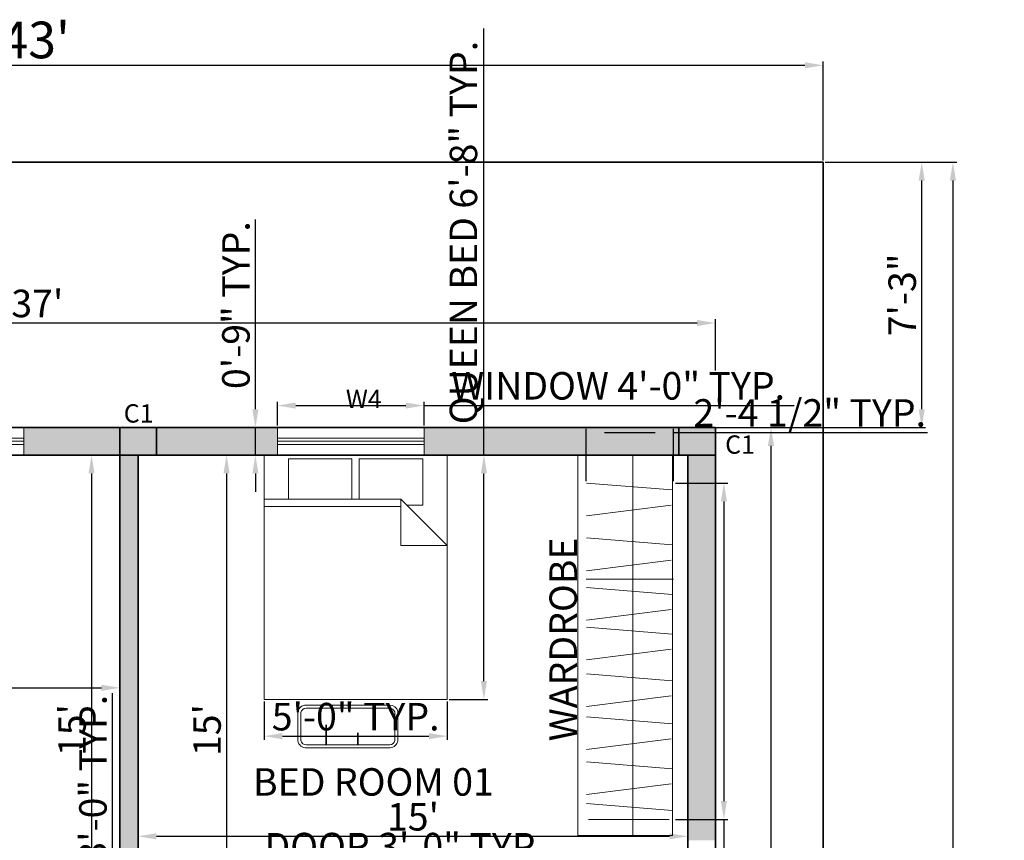
# Model space of a CAD drawing. Units: inches. Extents: x 4312 to 4955, y 6030 to 6717.
# Tile 5 of 5: x 4632 to 4955, y 6418 to 6686. Entities that reach past the tile are written whole.
import ezdxf

# ---------------------------------------------------------------- set-up
doc = ezdxf.new("R2010")
doc.units = ezdxf.units.IN
for name, color, linetype, lineweight in [('A-AREA-IDEN', 7, 'Continuous', 20), ('A-FLOR-CASE', 40, 'Continuous', 18), ('A-WALL', 7, 'Continuous', 35), ('C-PROP', 7, 'Continuous', 35), ('Dimensions', 112, 'Continuous', 13), ('Furniture', 30, 'Continuous', 18), ('Text', 30, 'Continuous', 18), ('Windows', 160, 'Continuous', 18)]:
    doc.layers.add(name, color=color, linetype=linetype, lineweight=lineweight)
doc.layers.add('A-WALL-PATT', color=251, linetype='Continuous', lineweight=13, true_color=0x636466)
doc.layers.add('Column', color=52, linetype='Continuous', lineweight=35, true_color=0xc8c92d)
doc.styles.get("Standard").update_dxf_attribs({"font": 'arial.ttf'})
doc.dimstyles.new('ISO-25', dxfattribs={"dimtxt": 9, "dimasz": 6, "dimexe": 1.25, "dimexo": 0.625, "dimtad": 1, "dimdec": 1, "dimlunit": 3, "dimtxsty": 'Standard', "dimcen": 2.5, "dimadec": 0, "dimazin": 0, "dimtfac": 1, "dimtdec": 1, "dimtmove": 0, "dimatfit": 3, "dimfxl": 1, "dimarcsym": 0})

# ---------------------------------------------------------------- blocks, each defined once
blk = doc.blocks.new('W')
at = {"layer": 'Windows'}
for p, q in [((4457.75, 6177.72), (4457.75, 6168.72)), ((4505.75, 6177.72), (4505.75, 6168.72)), ((4457.75, 6174.22), (4505.75, 6174.22)), ((4457.75, 6173.22), (4505.75, 6173.22)), ((4457.75, 6172.22), (4505.75, 6172.22))]:
    blk.add_line(p, q, dxfattribs=at)
blk = doc.blocks.new('*D11')
at = {"layer": 'Defpoints', "color": 0, "transparency": 16777216}
for p in [(4551.05, 6471.59), (4665.05, 6471.59), (4665.05, 6467.55)]:
    blk.add_point(p, dxfattribs=at)
at = {"layer": 'Dimensions', "color": 0, "lineweight": -2, "transparency": 16777216}
for p, q in [((4551.05, 6470.96), (4551.05, 6466.3)), ((4665.05, 6470.96), (4665.05, 6466.3)), ((4557.05, 6467.55), (4659.05, 6467.55))]:
    blk.add_line(p, q, dxfattribs=at)
at = {"layer": 'Dimensions', "color": 0, "transparency": 16777216}
for points in [[(4557.05, 6468.55), (4557.05, 6466.55), (4551.05, 6467.55)], [(4659.05, 6468.55), (4659.05, 6466.55), (4665.05, 6467.55)]]:
    blk.add_solid(points, dxfattribs=at)
at = {"layer": 'Dimensions', "color": 0, "transparency": 16777216, "insert": (4608.05, 6472.77), "char_height": 9, "attachment_point": 5}
blk.add_mtext('9\'-6"', dxfattribs=at)
blk = doc.blocks.new('*D12')
at = {"layer": 'Defpoints', "color": 0, "transparency": 16777216}
for p in [(4655.8, 6543.72), (4655.8, 6363.72), (4665.05, 6363.72)]:
    blk.add_point(p, dxfattribs=at)
at = {"layer": 'Dimensions', "color": 0, "lineweight": -2, "transparency": 16777216}
for p, q in [((4656.43, 6543.72), (4657.05, 6543.72)), ((4655.8, 6537.72), (4655.8, 6369.72)), ((4664.42, 6363.72), (4654.55, 6363.72))]:
    blk.add_line(p, q, dxfattribs=at)
at = {"layer": 'Dimensions', "color": 0, "transparency": 16777216}
for points in [[(4654.8, 6537.72), (4656.8, 6537.72), (4655.8, 6543.72)], [(4654.8, 6369.72), (4656.8, 6369.72), (4655.8, 6363.72)]]:
    blk.add_solid(points, dxfattribs=at)
at = {"layer": 'Dimensions', "color": 0, "transparency": 16777216, "insert": (4650.58, 6453.72), "char_height": 9, "attachment_point": 5, "rotation": 90}
blk.add_mtext("15'", dxfattribs=at)
blk = doc.blocks.new('*D13')
at = {"layer": 'Defpoints', "color": 0, "transparency": 16777216}
for p in [(4690.28, 6543.72), (4690.28, 6363.72), (4700.01, 6363.72)]:
    blk.add_point(p, dxfattribs=at)
at = {"layer": 'Dimensions', "color": 0, "lineweight": -2, "transparency": 16777216}
for p, q in [((4690.91, 6543.72), (4701.26, 6543.72)), ((4700.01, 6537.72), (4700.01, 6369.72)), ((4690.91, 6363.72), (4701.26, 6363.72))]:
    blk.add_line(p, q, dxfattribs=at)
at = {"layer": 'Dimensions', "color": 0, "transparency": 16777216}
for points in [[(4699.01, 6537.72), (4701.01, 6537.72), (4700.01, 6543.72)], [(4699.01, 6369.72), (4701.01, 6369.72), (4700.01, 6363.72)]]:
    blk.add_solid(points, dxfattribs=at)
at = {"layer": 'Dimensions', "color": 0, "transparency": 16777216, "insert": (4694.79, 6453.72), "char_height": 9, "attachment_point": 5, "rotation": 90}
blk.add_mtext("15'", dxfattribs=at)
blk = doc.blocks.new('*D14')
at = {"layer": 'Defpoints', "color": 0, "transparency": 16777216}
for p in [(4671.05, 6418.94), (4851.05, 6418.94), (4851.05, 6418.94)]:
    blk.add_point(p, dxfattribs=at)
at = {"layer": 'Dimensions', "color": 0, "lineweight": -2, "transparency": 16777216}
for p, q in [((4671.05, 6419.56), (4671.05, 6420.19)), ((4677.05, 6418.94), (4845.05, 6418.94)), ((4851.05, 6419.56), (4851.05, 6420.19))]:
    blk.add_line(p, q, dxfattribs=at)
at = {"layer": 'Dimensions', "color": 0, "transparency": 16777216}
for points in [[(4677.05, 6419.94), (4677.05, 6417.94), (4671.05, 6418.94)], [(4845.05, 6419.94), (4845.05, 6417.94), (4851.05, 6418.94)]]:
    blk.add_solid(points, dxfattribs=at)
at = {"layer": 'Dimensions', "color": 0, "transparency": 16777216, "insert": (4761.05, 6424.16), "char_height": 9, "attachment_point": 5}
blk.add_mtext("15'", dxfattribs=at)
blk = doc.blocks.new('*D38')
at = {"layer": 'Defpoints', "color": 0, "transparency": 16777216}
for p in [(4860.05, 6586.94), (4416.05, 6570.77), (4860.05, 6570.77)]:
    blk.add_point(p, dxfattribs=at)
at = {"layer": 'Dimensions', "color": 0, "lineweight": -2, "transparency": 16777216}
for p, q in [((4416.05, 6571.39), (4416.05, 6588.19)), ((4422.05, 6586.94), (4854.05, 6586.94)), ((4860.05, 6571.39), (4860.05, 6588.19))]:
    blk.add_line(p, q, dxfattribs=at)
at = {"layer": 'Dimensions', "color": 0, "transparency": 16777216}
for points in [[(4422.05, 6587.94), (4422.05, 6585.94), (4416.05, 6586.94)], [(4854.05, 6587.94), (4854.05, 6585.94), (4860.05, 6586.94)]]:
    blk.add_solid(points, dxfattribs=at)
at = {"layer": 'Dimensions', "color": 0, "transparency": 16777216, "insert": (4638.05, 6592.16), "char_height": 9, "attachment_point": 5}
blk.add_mtext("37'", dxfattribs=at)
blk = doc.blocks.new('*D39')
at = {"layer": 'Defpoints', "color": 0, "transparency": 16777216}
for p in [(4857.98, 6552.72), (4864.3, 6168.72), (4878.26, 6168.72)]:
    blk.add_point(p, dxfattribs=at)
at = {"layer": 'Dimensions', "color": 0, "lineweight": -2, "transparency": 16777216}
for p, q in [((4858.6, 6552.72), (4879.51, 6552.72)), ((4878.26, 6546.72), (4878.26, 6174.72)), ((4864.93, 6168.72), (4879.51, 6168.72))]:
    blk.add_line(p, q, dxfattribs=at)
at = {"layer": 'Dimensions', "color": 0, "transparency": 16777216}
for points in [[(4877.26, 6546.72), (4879.26, 6546.72), (4878.26, 6552.72)], [(4877.26, 6174.72), (4879.26, 6174.72), (4878.26, 6168.72)]]:
    blk.add_solid(points, dxfattribs=at)
at = {"layer": 'Dimensions', "color": 0, "transparency": 16777216, "insert": (4873.03, 6360.72), "char_height": 9, "attachment_point": 5, "rotation": 90}
blk.add_mtext("32'", dxfattribs=at)
blk = doc.blocks.new('*D40')
at = {"layer": 'Defpoints', "color": 0, "transparency": 16777216}
for p in [(4895.36, 6671.27), (4379.36, 6639.55), (4895.36, 6639.55)]:
    blk.add_point(p, dxfattribs=at)
at = {"layer": 'Dimensions', "color": 0, "lineweight": -2, "transparency": 16777216}
for p, q in [((4379.36, 6640.17), (4379.36, 6672.52)), ((4385.36, 6671.27), (4889.36, 6671.27)), ((4895.36, 6640.17), (4895.36, 6672.52))]:
    blk.add_line(p, q, dxfattribs=at)
at = {"layer": 'Dimensions', "color": 0, "transparency": 16777216}
for points in [[(4385.36, 6672.27), (4385.36, 6670.27), (4379.36, 6671.27)], [(4889.36, 6672.27), (4889.36, 6670.27), (4895.36, 6671.27)]]:
    blk.add_solid(points, dxfattribs=at)
at = {"layer": 'Dimensions', "color": 0, "transparency": 16777216, "insert": (4637.36, 6678.02), "char_height": 12, "attachment_point": 5}
blk.add_mtext("43'", dxfattribs=at)
blk = doc.blocks.new('*D41')
at = {"layer": 'Defpoints', "color": 0, "transparency": 16777216}
for p in [(4895.36, 6639.55), (4895.36, 6070.55), (4937.83, 6070.55)]:
    blk.add_point(p, dxfattribs=at)
at = {"layer": 'Dimensions', "color": 0, "lineweight": -2, "transparency": 16777216}
for p, q in [((4895.99, 6639.55), (4939.08, 6639.55)), ((4937.83, 6633.55), (4937.83, 6076.55)), ((4895.99, 6070.55), (4939.08, 6070.55))]:
    blk.add_line(p, q, dxfattribs=at)
at = {"layer": 'Dimensions', "color": 0, "transparency": 16777216}
for points in [[(4936.83, 6633.55), (4938.83, 6633.55), (4937.83, 6639.55)], [(4936.83, 6076.55), (4938.83, 6076.55), (4937.83, 6070.55)]]:
    blk.add_solid(points, dxfattribs=at)
at = {"layer": 'Dimensions', "color": 0, "transparency": 16777216, "insert": (4931.11, 6355.05), "char_height": 12, "attachment_point": 5, "rotation": 90}
blk.add_mtext('47\'-5"', dxfattribs=at)
blk = doc.blocks.new('BED-QUEEN-PLAN')
for p, q in [((0, 0), (0, 80.00003)), ((7.99999, 78.80003), (28.79998, 78.80003)), ((7.99999, 65.60003), (7.99999, 78.80003)), ((28.79998, 78.80003), (28.79998, 65.60003)), ((31.19999, 78.80003), (51.99999, 78.80003)), ((31.19999, 65.60003), (31.19999, 78.80003)), ((51.99999, 78.80003), (51.99999, 63.60003)), ((59.99999, 80.00003), (59.99999, 0)), ((0, 65.60003), (44.8, 65.60003)), ((59.99999, 50.40003), (44.8, 65.60003)), ((44.8, 65.60003), (44.8, 50.40003)), ((44.8, 63.20003), (0, 63.20003)), ((51.99999, 63.60003), (46.79936, 63.60003)), ((44.8, 50.40003), (59.99999, 50.40003)), ((59.99999, 0), (0, 0))]:
    blk.add_line(p, q)
blk = doc.blocks.new('BEDROOM-BENCH')
for p, q in [((9.25, 1.01), (9.25, 7.57)), ((9.35, 1.01), (9.35, 7.57)), ((9.45, 1.01), (9.45, 7.57)), ((19.62, 1.01), (19.62, 4.91)), ((19.72, 1.01), (19.72, 4.91)), ((19.82, 1.01), (19.82, 4.91))]:
    blk.add_line(p, q)
blk.add_lwpolyline([(30.1, 13.99), (2.75, 13.99, 0.367048), (0, 11.66), (0, 2.33, 0.386896), (2.94, 0.01), (30.22, 0.01, 0.350808), (32.79, 2.35), (32.79, 11.9, 0.341474)], format="xyb", close=True)
blk.add_lwpolyline([(30.1, 12.99), (2.75, 12.99, 0.355496), (1, 11.56), (1, 2.42, 0.38014), (2.9, 1.01), (30.18, 1.01, 0.335385), (31.79, 2.44), (31.79, 11.76, 0.335385), (30.02, 12.99)], format="xyb")
blk = doc.blocks.new('WARDROBE-HANGING-RAIL')
for p, q in [((0, 0.04), (2.27, 28.16)), ((7.23, 27.75), (10.74, 0.04)), ((17.98, 0.04), (20.26, 28.16)), ((25.22, 27.75), (28.73, 0.04)), ((31.43, 0), (31.43, 28.54)), ((34.18, 0.04), (36.45, 28.16)), ((41.41, 27.75), (44.92, 0.04)), ((47.17, 0.04), (49.44, 28.16)), ((54.4, 27.75), (57.91, 0.04)), ((62.41, 0.04), (64.68, 28.16)), ((69.64, 27.75), (73.15, 0.04)), ((76.5, 0.04), (78.77, 28.16)), ((83.73, 27.75), (87.24, 0.04)), ((91.21, 0.04), (93.48, 28.16)), ((98.44, 27.75), (101.95, 0.04)), ((104.86, 0.04), (107.13, 28.16)), ((110.06, 27.17), (110.06, 0.69))]:
    blk.add_line(p, q)
blk = doc.blocks.new('COLUMN-12X9-INLINE')
h = blk.add_hatch(color=256)
h.dxf.hatch_style = 1
h.paths.add_polyline_path([(12, 0), (12, 9), (0, 9), (0, 0)])
for points in [[(0, 0), (0, 9)], [(12, 9), (12, 0)]]:
    blk.add_lwpolyline(points)
blk = doc.blocks.new('*D57')
at = {"layer": 'Defpoints', "color": 0, "transparency": 16777216}
for p in [(4764.66, 6559.92), (4716.66, 6552.72), (4764.66, 6552.72)]:
    blk.add_point(p, dxfattribs=at)
at = {"layer": 'Dimensions', "color": 0, "lineweight": -2, "transparency": 16777216}
for p, q in [((4716.66, 6553.35), (4716.66, 6561.17)), ((4764.66, 6553.35), (4764.66, 6561.17)), ((4722.66, 6559.92), (4758.66, 6559.92)), ((4764.66, 6559.92), (4885.8, 6559.92))]:
    blk.add_line(p, q, dxfattribs=at)
at = {"layer": 'Dimensions', "color": 0, "transparency": 16777216}
for points in [[(4722.66, 6560.92), (4722.66, 6558.92), (4716.66, 6559.92)], [(4758.66, 6560.92), (4758.66, 6558.92), (4764.66, 6559.92)]]:
    blk.add_solid(points, dxfattribs=at)
at = {"layer": 'Dimensions', "color": 0, "transparency": 16777216, "insert": (4828.23, 6565.21), "char_height": 9, "attachment_point": 5}
blk.add_mtext('WINDOW 4\'-0" TYP.', dxfattribs=at)
blk = doc.blocks.new('*D58')
at = {"layer": 'Defpoints', "color": 0, "transparency": 16777216}
for p in [(4709.46, 6552.72), (4716.66, 6552.72), (4716.66, 6543.72)]:
    blk.add_point(p, dxfattribs=at)
at = {"layer": 'Dimensions', "color": 0, "lineweight": -2, "transparency": 16777216}
for p, q in [((4709.46, 6558.72), (4709.46, 6620.83)), ((4716.03, 6552.72), (4708.21, 6552.72)), ((4709.46, 6543.72), (4709.46, 6552.72)), ((4716.03, 6543.72), (4708.21, 6543.72)), ((4709.46, 6537.72), (4709.46, 6531.72))]:
    blk.add_line(p, q, dxfattribs=at)
at = {"layer": 'Dimensions', "color": 0, "transparency": 16777216}
for points in [[(4708.46, 6558.72), (4710.46, 6558.72), (4709.46, 6552.72)], [(4708.46, 6537.72), (4710.46, 6537.72), (4709.46, 6543.72)]]:
    blk.add_solid(points, dxfattribs=at)
at = {"layer": 'Dimensions', "color": 0, "transparency": 16777216, "insert": (4704.24, 6592.78), "char_height": 9, "attachment_point": 5, "rotation": 90}
blk.add_mtext('0\'-9" TYP.', dxfattribs=at)
blk = doc.blocks.new('*D59')
at = {"layer": 'Defpoints', "color": 0, "transparency": 16777216}
for p in [(4704.05, 6409.12), (4668.05, 6403.72), (4704.05, 6403.72)]:
    blk.add_point(p, dxfattribs=at)
at = {"layer": 'Dimensions', "color": 0, "lineweight": -2, "transparency": 16777216}
for p, q in [((4668.05, 6404.35), (4668.05, 6410.37)), ((4674.05, 6409.12), (4698.05, 6409.12)), ((4704.05, 6404.35), (4704.05, 6410.37)), ((4704.05, 6409.12), (4806.92, 6409.12))]:
    blk.add_line(p, q, dxfattribs=at)
at = {"layer": 'Dimensions', "color": 0, "transparency": 16777216}
for points in [[(4674.05, 6410.12), (4674.05, 6408.12), (4668.05, 6409.12)], [(4698.05, 6410.12), (4698.05, 6408.12), (4704.05, 6409.12)]]:
    blk.add_solid(points, dxfattribs=at)
at = {"layer": 'Dimensions', "color": 0, "transparency": 16777216, "insert": (4758.49, 6414.41), "char_height": 9, "attachment_point": 5}
blk.add_mtext('DOOR 3\'-0" TYP.', dxfattribs=at)
blk = doc.blocks.new('*D60')
at = {"layer": 'Defpoints', "color": 0, "transparency": 16777216}
for p in [(4662.65, 6403.72), (4668.05, 6403.72), (4668.05, 6367.72)]:
    blk.add_point(p, dxfattribs=at)
at = {"layer": 'Dimensions', "color": 0, "lineweight": -2, "transparency": 16777216}
for p, q in [((4662.65, 6403.72), (4662.65, 6465.83)), ((4667.42, 6403.72), (4661.4, 6403.72)), ((4662.65, 6373.72), (4662.65, 6397.72)), ((4667.42, 6367.72), (4661.4, 6367.72))]:
    blk.add_line(p, q, dxfattribs=at)
at = {"layer": 'Dimensions', "color": 0, "transparency": 16777216}
for points in [[(4661.65, 6397.72), (4663.65, 6397.72), (4662.65, 6403.72)], [(4661.65, 6373.72), (4663.65, 6373.72), (4662.65, 6367.72)]]:
    blk.add_solid(points, dxfattribs=at)
at = {"layer": 'Dimensions', "color": 0, "transparency": 16777216, "insert": (4657.43, 6437.78), "char_height": 9, "attachment_point": 5, "rotation": 90}
blk.add_mtext('3\'-0" TYP.', dxfattribs=at)
blk = doc.blocks.new('*D71')
at = {"layer": 'Defpoints', "color": 0, "transparency": 16777216}
for p in [(4772.28, 6543.72), (4784.28, 6543.72), (4772.28, 6463.72)]:
    blk.add_point(p, dxfattribs=at)
at = {"layer": 'Dimensions', "color": 0, "lineweight": -2, "transparency": 16777216}
for p, q in [((4784.28, 6543.72), (4784.28, 6683.37)), ((4772.9, 6543.72), (4785.53, 6543.72)), ((4784.28, 6469.72), (4784.28, 6537.72)), ((4772.9, 6463.72), (4785.53, 6463.72))]:
    blk.add_line(p, q, dxfattribs=at)
at = {"layer": 'Dimensions', "color": 0, "transparency": 16777216}
for points in [[(4783.28, 6537.72), (4785.28, 6537.72), (4784.28, 6543.72)], [(4783.28, 6469.72), (4785.28, 6469.72), (4784.28, 6463.72)]]:
    blk.add_solid(points, dxfattribs=at)
at = {"layer": 'Dimensions', "color": 0, "transparency": 16777216, "insert": (4778.72, 6616.54), "char_height": 9, "attachment_point": 5, "rotation": 90}
blk.add_mtext('QUEEN BED 6\'-8" TYP.', dxfattribs=at)
blk = doc.blocks.new('*D72')
at = {"layer": 'Defpoints', "color": 0, "transparency": 16777216}
for p in [(4712.28, 6463.72), (4772.28, 6463.72), (4772.28, 6451.72)]:
    blk.add_point(p, dxfattribs=at)
at = {"layer": 'Dimensions', "color": 0, "lineweight": -2, "transparency": 16777216}
for p, q in [((4712.28, 6463.1), (4712.28, 6450.47)), ((4772.28, 6463.1), (4772.28, 6450.47)), ((4718.28, 6451.72), (4766.28, 6451.72))]:
    blk.add_line(p, q, dxfattribs=at)
at = {"layer": 'Dimensions', "color": 0, "transparency": 16777216}
for points in [[(4718.28, 6452.72), (4718.28, 6450.72), (4712.28, 6451.72)], [(4766.28, 6452.72), (4766.28, 6450.72), (4772.28, 6451.72)]]:
    blk.add_solid(points, dxfattribs=at)
at = {"layer": 'Dimensions', "color": 0, "transparency": 16777216, "insert": (4742.28, 6456.94), "char_height": 9, "attachment_point": 5}
blk.add_mtext('5\'-0" TYP.', dxfattribs=at)
blk = doc.blocks.new('*D79')
at = {"layer": 'Defpoints', "color": 0, "transparency": 16777216}
for p in [(4846.33, 6534.56), (4846.33, 6424.5), (4862.84, 6424.5)]:
    blk.add_point(p, dxfattribs=at)
at = {"layer": 'Dimensions', "color": 0, "lineweight": -2, "transparency": 16777216}
for p, q in [((4846.95, 6534.56), (4864.09, 6534.56)), ((4862.84, 6528.56), (4862.84, 6430.5)), ((4846.95, 6424.5), (4864.09, 6424.5)), ((4862.84, 6424.5), (4862.84, 6284.48))]:
    blk.add_line(p, q, dxfattribs=at)
at = {"layer": 'Dimensions', "color": 0, "transparency": 16777216}
for points in [[(4861.84, 6528.56), (4863.84, 6528.56), (4862.84, 6534.56)], [(4861.84, 6430.5), (4863.84, 6430.5), (4862.84, 6424.5)]]:
    blk.add_solid(points, dxfattribs=at)
at = {"layer": 'Dimensions', "color": 0, "transparency": 16777216, "insert": (4857.56, 6351.49), "char_height": 9, "attachment_point": 5, "rotation": 90}
blk.add_mtext('WARDROBE 9\'-2" TYP.', dxfattribs=at)
blk = doc.blocks.new('*D80')
at = {"layer": 'Defpoints', "color": 0, "transparency": 16777216}
for p in [(4846.33, 6551.06), (4817.79, 6534.56), (4846.33, 6534.56)]:
    blk.add_point(p, dxfattribs=at)
at = {"layer": 'Dimensions', "color": 0, "lineweight": -2, "transparency": 16777216}
for p, q in [((4817.79, 6535.18), (4817.79, 6552.31)), ((4823.79, 6551.06), (4840.33, 6551.06)), ((4846.33, 6535.18), (4846.33, 6552.31)), ((4846.33, 6551.06), (4929.56, 6551.06))]:
    blk.add_line(p, q, dxfattribs=at)
at = {"layer": 'Dimensions', "color": 0, "transparency": 16777216}
for points in [[(4823.79, 6552.06), (4823.79, 6550.06), (4817.79, 6551.06)], [(4840.33, 6552.06), (4840.33, 6550.06), (4846.33, 6551.06)]]:
    blk.add_solid(points, dxfattribs=at)
at = {"layer": 'Dimensions', "color": 0, "transparency": 16777216, "insert": (4890.95, 6556.34), "char_height": 9, "attachment_point": 5}
blk.add_mtext('2\'-4 1/2" TYP.', dxfattribs=at)
blk = doc.blocks.new('*D87')
at = {"layer": 'Defpoints', "color": 0, "transparency": 16777216}
for p in [(4895.36, 6639.55), (4927.61, 6639.55), (4860.05, 6552.72)]:
    blk.add_point(p, dxfattribs=at)
at = {"layer": 'Dimensions', "color": 0, "lineweight": -2, "transparency": 16777216}
for p, q in [((4895.99, 6639.55), (4928.86, 6639.55)), ((4927.61, 6558.72), (4927.61, 6633.55)), ((4860.67, 6552.72), (4928.86, 6552.72))]:
    blk.add_line(p, q, dxfattribs=at)
at = {"layer": 'Dimensions', "color": 0, "transparency": 16777216}
for points in [[(4926.61, 6633.55), (4928.61, 6633.55), (4927.61, 6639.55)], [(4926.61, 6558.72), (4928.61, 6558.72), (4927.61, 6552.72)]]:
    blk.add_solid(points, dxfattribs=at)
at = {"layer": 'Dimensions', "color": 0, "transparency": 16777216, "insert": (4922.39, 6596.14), "char_height": 9, "attachment_point": 5, "rotation": 90}
blk.add_mtext('7\'-3"', dxfattribs=at)
blk = doc.blocks.new('*D88')
at = {"layer": 'Defpoints', "color": 0, "transparency": 16777216}
for p in [(4895.36, 6639.55), (4860.05, 6552.72), (4895.36, 6038.3)]:
    blk.add_point(p, dxfattribs=at)
at = {"layer": 'Dimensions', "color": 0, "lineweight": -2, "transparency": 16777216}
for p, q in [((4895.36, 6638.92), (4895.36, 6037.05)), ((4860.05, 6552.1), (4860.05, 6037.05)), ((4866.05, 6038.3), (4889.36, 6038.3)), ((4895.36, 6038.3), (4954.65, 6038.3))]:
    blk.add_line(p, q, dxfattribs=at)
at = {"layer": 'Dimensions', "color": 0, "transparency": 16777216}
for points in [[(4866.05, 6039.3), (4866.05, 6037.3), (4860.05, 6038.3)], [(4889.36, 6039.3), (4889.36, 6037.3), (4895.36, 6038.3)]]:
    blk.add_solid(points, dxfattribs=at)
at = {"layer": 'Dimensions', "color": 0, "transparency": 16777216, "insert": (4928.01, 6043.58), "char_height": 9, "attachment_point": 5}
blk.add_mtext('2\'-11 1/2"', dxfattribs=at)

msp = doc.modelspace()

# ---------------------------------------------------------------- hatches: boundary and pattern name
at = {"layer": 'A-WALL-PATT'}
h = msp.add_hatch(color=256, dxfattribs=at)
h.dxf.hatch_style = 1
h.paths.add_polyline_path([(4665.05, 6552.72), (4633.64, 6552.72), (4633.64, 6543.72), (4665.05, 6543.72)])
h = msp.add_hatch(color=256, dxfattribs=at)
h.dxf.hatch_style = 1
h.paths.add_polyline_path([(4716.66, 6552.72), (4677.05, 6552.72), (4677.05, 6543.72), (4716.66, 6543.72)])
h = msp.add_hatch(color=256, dxfattribs=at)
h.dxf.hatch_style = 1
h.paths.add_polyline_path([(4848.05, 6552.72), (4764.66, 6552.72), (4764.66, 6543.72), (4848.05, 6543.72)])
h = msp.add_hatch(color=256, dxfattribs=at)
h.dxf.hatch_style = 1
h.paths.add_polyline_path([(4671.05, 6543.72), (4665.05, 6543.72), (4665.05, 6403.72), (4671.05, 6403.72)])
h = msp.add_hatch(color=256, dxfattribs=at)
h.dxf.hatch_style = 1
h.paths.add_polyline_path([(4860.05, 6543.72), (4851.05, 6543.72), (4851.05, 6417.64), (4860.05, 6417.64)])
at = {"layer": 'Column'}
h = msp.add_hatch(color=256, dxfattribs=at)
h.dxf.hatch_style = 1
h.paths.add_polyline_path([(4860.05, 6543.72), (4860.05, 6552.72), (4848.05, 6552.72), (4848.05, 6543.72)])

# ---------------------------------------------------------------- linework, layer by layer
at = {"layer": 'A-FLOR-CASE'}
for p, q in [((4815.05, 6543.72), (4815.05, 6419.25)), ((4833.05, 6419.25), (4833.05, 6543.72)), ((4846.06, 6543.72), (4846.06, 6419.25)), ((4846.06, 6419.25), (4815.05, 6419.25))]:
    msp.add_line(p, q, dxfattribs=at)
at = {"layer": 'A-WALL'}
for p, q in [((4416.05, 6552.72), (4860.05, 6552.72)), ((4860.05, 6552.72), (4860.05, 6090.72)), ((4551.05, 6543.72), (4851.05, 6543.72)), ((4665.05, 6543.72), (4665.05, 6403.72)), ((4671.05, 6543.72), (4671.05, 6403.72)), ((4851.05, 6543.72), (4851.05, 6270.72))]:
    msp.add_line(p, q, dxfattribs=at)
at = {"layer": 'C-PROP'}
msp.add_lwpolyline([(4895.36, 6639.55), (4895.36, 6070.55), (4355.36, 6070.55), (4379.36, 6639.55)], close=True, dxfattribs=at)
at = {"layer": 'Column'}
msp.add_lwpolyline([(4860.05, 6543.72), (4848.05, 6543.72), (4848.05, 6552.72)], dxfattribs=at)
at = {"layer": 'Furniture'}
msp.add_line((4772.28, 6482.13), (4772.28, 6482.13), dxfattribs=at)

# ---------------------------------------------------------------- block references
at = {"layer": 'A-FLOR-CASE', "rotation": 270.0000000000004}
msp.add_blockref('WARDROBE-HANGING-RAIL', (4817.79, 6534.56), dxfattribs=at)
at = {"layer": 'Column'}
msp.add_blockref('COLUMN-12X9-INLINE', (4665.05, 6543.72), dxfattribs=at)
at = {"layer": 'Furniture'}
for name, p in [('BED-QUEEN-PLAN', (4712.28, 6463.72)), ('BEDROOM-BENCH', (4723.31, 6447.89))]:
    msp.add_blockref(name, p, dxfattribs=at)
at = {"layer": 'Windows'}
for p in [(127.88, 375), (258.91, 375)]:
    msp.add_blockref('W', p, dxfattribs=at)

# ---------------------------------------------------------------- texts
at = {"layer": 'A-AREA-IDEN', "insert": (4708.66, 6441.24), "char_height": 9, "attachment_point": 1, "rotation": 0.0025}
msp.add_mtext_dynamic_manual_height_columns('BED ROOM 01', width=89.0701, gutter_width=12.5, heights=[0], dxfattribs=at)
at = {"layer": 'Text', "char_height": 6, "attachment_point": 1}
for s, insert in [('W4', (4739.07, 6565.08)), ('C1', (4666.34, 6560.35)), ('C1', (4863.25, 6550.15))]:
    msp.add_mtext_dynamic_manual_height_columns(s, width=4.4911, gutter_width=12.5, heights=[0], dxfattribs=dict(at, insert=insert))
at = {"layer": 'Text', "insert": (4805.74, 6450.05), "char_height": 9, "attachment_point": 1, "rotation": 90.0025}
msp.add_mtext_dynamic_manual_height_columns('WARDROBE', width=89.0701, gutter_width=12.5, heights=[0], dxfattribs=at)

# ---------------------------------------------------------------- dimensions: what is measured, and where the dimension line sits
at = {"layer": 'Dimensions'}
for base, p1, p2, override, picture, middle in [((4895.36, 6671.27), (4379.36, 6639.55), (4895.36, 6639.55), {"dimtxt": 12, "dimclrd": 0, "dimclre": 0, "dimclrt": 0}, '*D40', (4637.36, 6678.02)), ((4895.36, 6038.3), (4860.05, 6552.72), (4895.36, 6639.55), {"dimdec": 1, "dimlfac": 1, "dimrnd": 0, "dimzin": 1, "dimdsep": 46, "dimlunit": 4, "dimfrac": 2}, '*D88', (4928.01, 6043.58)), ((4860.05, 6586.94), (4416.05, 6570.77), (4860.05, 6570.77), {"dimclrd": 0, "dimclre": 0, "dimclrt": 0}, '*D38', (4638.05, 6592.16)), ((4665.05, 6467.55), (4551.05, 6471.59), (4665.05, 6471.59), {"dimclrd": 0, "dimclre": 0, "dimclrt": 0}, '*D11', (4608.05, 6472.77)), ((4851.05, 6418.94), (4671.05, 6418.94), (4851.05, 6418.94), {"dimclrd": 0, "dimclre": 0, "dimclrt": 0}, '*D14', (4761.05, 6424.16))]:
    dim = msp.add_linear_dim(base=base, p1=p1, p2=p2, dimstyle='ISO-25', override=override, dxfattribs=at)
    dim.commit()
    dim.dimension.update_dxf_attribs({"geometry": picture, "text_midpoint": middle})
for base, p1, p2, angle, text, picture, middle in [((4784.28, 6543.72), (4772.28, 6463.72), (4772.28, 6543.72), 90, 'QUEEN BED <> TYP.', '*D71', (4778.72, 6616.54)), ((4709.46, 6552.72), (4716.66, 6543.72), (4716.66, 6552.72), 90, '<> TYP.', '*D58', (4704.24, 6592.78)), ((4862.84, 6424.5), (4846.33, 6534.56), (4846.33, 6424.5), 270, 'WARDROBE <> TYP.', '*D79', (4857.56, 6351.49)), ((4662.65, 6403.72), (4668.05, 6367.72), (4668.05, 6403.72), 90, '<> TYP.', '*D60', (4657.43, 6437.78))]:
    dim = msp.add_linear_dim(base=base, p1=p1, p2=p2, angle=angle, text=text, dimstyle='ISO-25', override={"dimdec": 1, "dimlfac": 1, "dimrnd": 0, "dimzin": 1, "dimdsep": 46, "dimlunit": 4, "dimfrac": 2}, dxfattribs=at)
    dim.commit()
    dim.dimension.update_dxf_attribs({"geometry": picture, "text_midpoint": middle})
for base, p1, p2, override, picture, middle in [((4927.61, 6639.55), (4860.05, 6552.72), (4895.36, 6639.55), {"dimdec": 1, "dimlfac": 1, "dimrnd": 0, "dimzin": 1, "dimdsep": 46, "dimlunit": 4, "dimfrac": 2}, '*D87', (4922.39, 6596.14)), ((4937.83, 6070.55), (4895.36, 6639.55), (4895.36, 6070.55), {"dimtxt": 12, "dimclrd": 0, "dimclre": 0, "dimclrt": 0}, '*D41', (4931.11, 6355.05)), ((4878.26, 6168.72), (4857.98, 6552.72), (4864.3, 6168.72), {"dimclrd": 0, "dimclre": 0, "dimclrt": 0}, '*D39', (4873.03, 6360.72)), ((4655.8, 6363.72), (4655.8, 6543.72), (4665.05, 6363.72), {"dimclrd": 0, "dimclre": 0, "dimclrt": 0}, '*D12', (4650.58, 6453.72)), ((4700.01, 6363.72), (4690.28, 6543.72), (4690.28, 6363.72), {"dimclrd": 0, "dimclre": 0, "dimclrt": 0}, '*D13', (4694.79, 6453.72))]:
    dim = msp.add_linear_dim(base=base, p1=p1, p2=p2, angle=90, dimstyle='ISO-25', override=override, dxfattribs=at)
    dim.commit()
    dim.dimension.update_dxf_attribs({"geometry": picture, "text_midpoint": middle})
for base, p1, p2, text, picture, middle in [((4764.66, 6559.92), (4716.66, 6552.72), (4764.66, 6552.72), 'WINDOW <> TYP.', '*D57', (4828.23, 6565.21)), ((4846.33, 6551.06), (4817.79, 6534.56), (4846.33, 6534.56), '<> TYP.', '*D80', (4890.95, 6556.34)), ((4772.28, 6451.72), (4712.28, 6463.72), (4772.28, 6463.72), '<> TYP.', '*D72', (4742.28, 6456.94)), ((4704.05, 6409.12), (4668.05, 6403.72), (4704.05, 6403.72), 'DOOR <> TYP.', '*D59', (4758.49, 6414.41))]:
    dim = msp.add_linear_dim(base=base, p1=p1, p2=p2, text=text, dimstyle='ISO-25', override={"dimdec": 1, "dimlfac": 1, "dimrnd": 0, "dimzin": 1, "dimdsep": 46, "dimlunit": 4, "dimfrac": 2}, dxfattribs=at)
    dim.commit()
    dim.dimension.update_dxf_attribs({"geometry": picture, "text_midpoint": middle})

doc.saveas('drawing.dxf')
